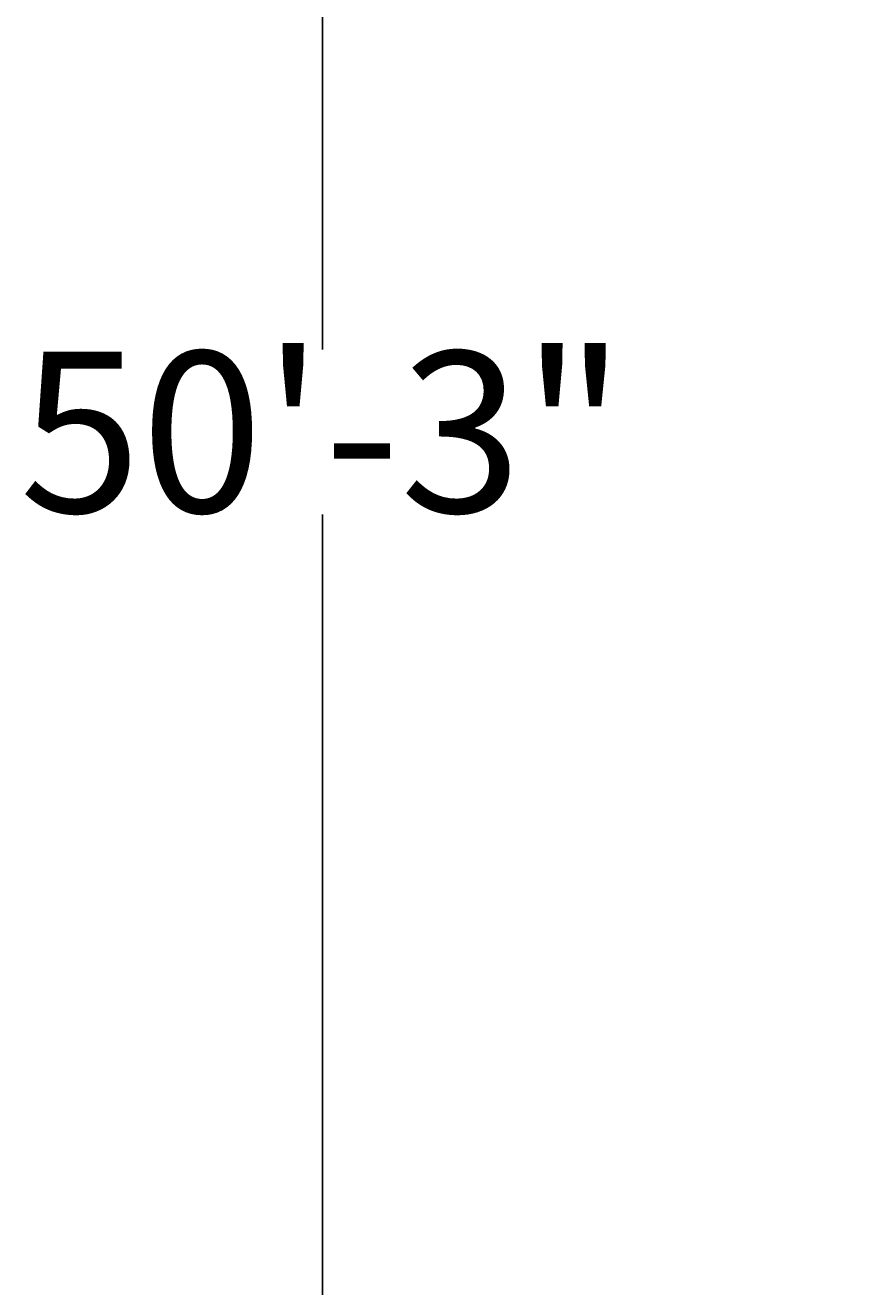
# Model space of a CAD drawing. Units: inches. Extents: x -304 to 580, y 363 to 1149.
# Tile 2 of 11: x -304 to -115, y 512 to 794. Entities that reach past the tile are written whole.
import ezdxf

# ---------------------------------------------------------------- set-up
doc = ezdxf.new("R2010")
doc.units = ezdxf.units.IN
doc.header["$MEASUREMENT"] = 0
doc.layers.add('A-ANNO-DIMS', color=2, linetype='Continuous', lineweight=13)
doc.styles.get("Standard").update_dxf_attribs({"font": 'arial.ttf'})
doc.dimstyles.get("Standard").update_dxf_attribs({"dimtxt": 1, "dimasz": 1, "dimexe": 0.18, "dimexo": 0.0625, "dimgap": 0.09, "dimtad": 0, "dimtih": 1, "dimtoh": 1, "dimdec": 0, "dimzin": 0, "dimdsep": 46, "dimlunit": 3, "dimtxsty": 'Standard', "dimcen": 0.09, "dimadec": 0, "dimazin": 0, "dimtfac": 1, "dimtdec": 0, "dimtofl": 0, "dimtmove": 0, "dimatfit": 3, "dimfxl": 1, "dimtolj": 1, "dimtzin": 0, "dimarcsym": 0})

# ---------------------------------------------------------------- blocks, each defined once
blk = doc.blocks.new('*D1')
at = {"layer": 'A-ANNO-DIMS', "color": 0, "lineweight": -2, "transparency": 16777216}
for p, q in [((-22.63, 1004.95), (-237.62, 1004.95)), ((-237.44, 1003.95), (-237.44, 721.93)), ((-237.44, 402.95), (-237.44, 684.96)), ((-22.63, 401.95), (-237.62, 401.95))]:
    blk.add_line(p, q, dxfattribs=at)
at = {"layer": 'A-ANNO-DIMS', "color": 0, "transparency": 16777216}
for points in [[(-237.61, 1003.95), (-237.28, 1003.95), (-237.44, 1004.95)], [(-237.61, 402.95), (-237.28, 402.95), (-237.44, 401.95)]]:
    blk.add_solid(points, dxfattribs=at)
at = {"layer": 'Defpoints', "color": 0, "transparency": 16777216}
for p in [(-22.57, 1004.95), (-237.44, 401.95), (-22.57, 401.95)]:
    blk.add_point(p, dxfattribs=at)
at = {"layer": 'A-ANNO-DIMS', "color": 0, "transparency": 16777216, "insert": (-237.44, 703.45), "char_height": 1, "attachment_point": 5}
blk.add_mtext('\\A1;{\\H36x;50\'-3"}', dxfattribs=at)

msp = doc.modelspace()

# ---------------------------------------------------------------- dimensions: what is measured, and where the dimension line sits
at = {"layer": 'A-ANNO-DIMS'}
dim = msp.add_linear_dim(base=(-237.44, 401.95), p1=(-22.57, 1004.95), p2=(-22.57, 401.95), angle=90, text='{\\H36x;<>}', dimstyle='Standard', override={"dimclrd": 0, "dimclre": 0, "dimclrt": 0}, dxfattribs=at)
dim.commit()
dim.dimension.update_dxf_attribs({"geometry": '*D1', "text_midpoint": (-237.44, 703.45)})

doc.saveas('drawing.dxf')
